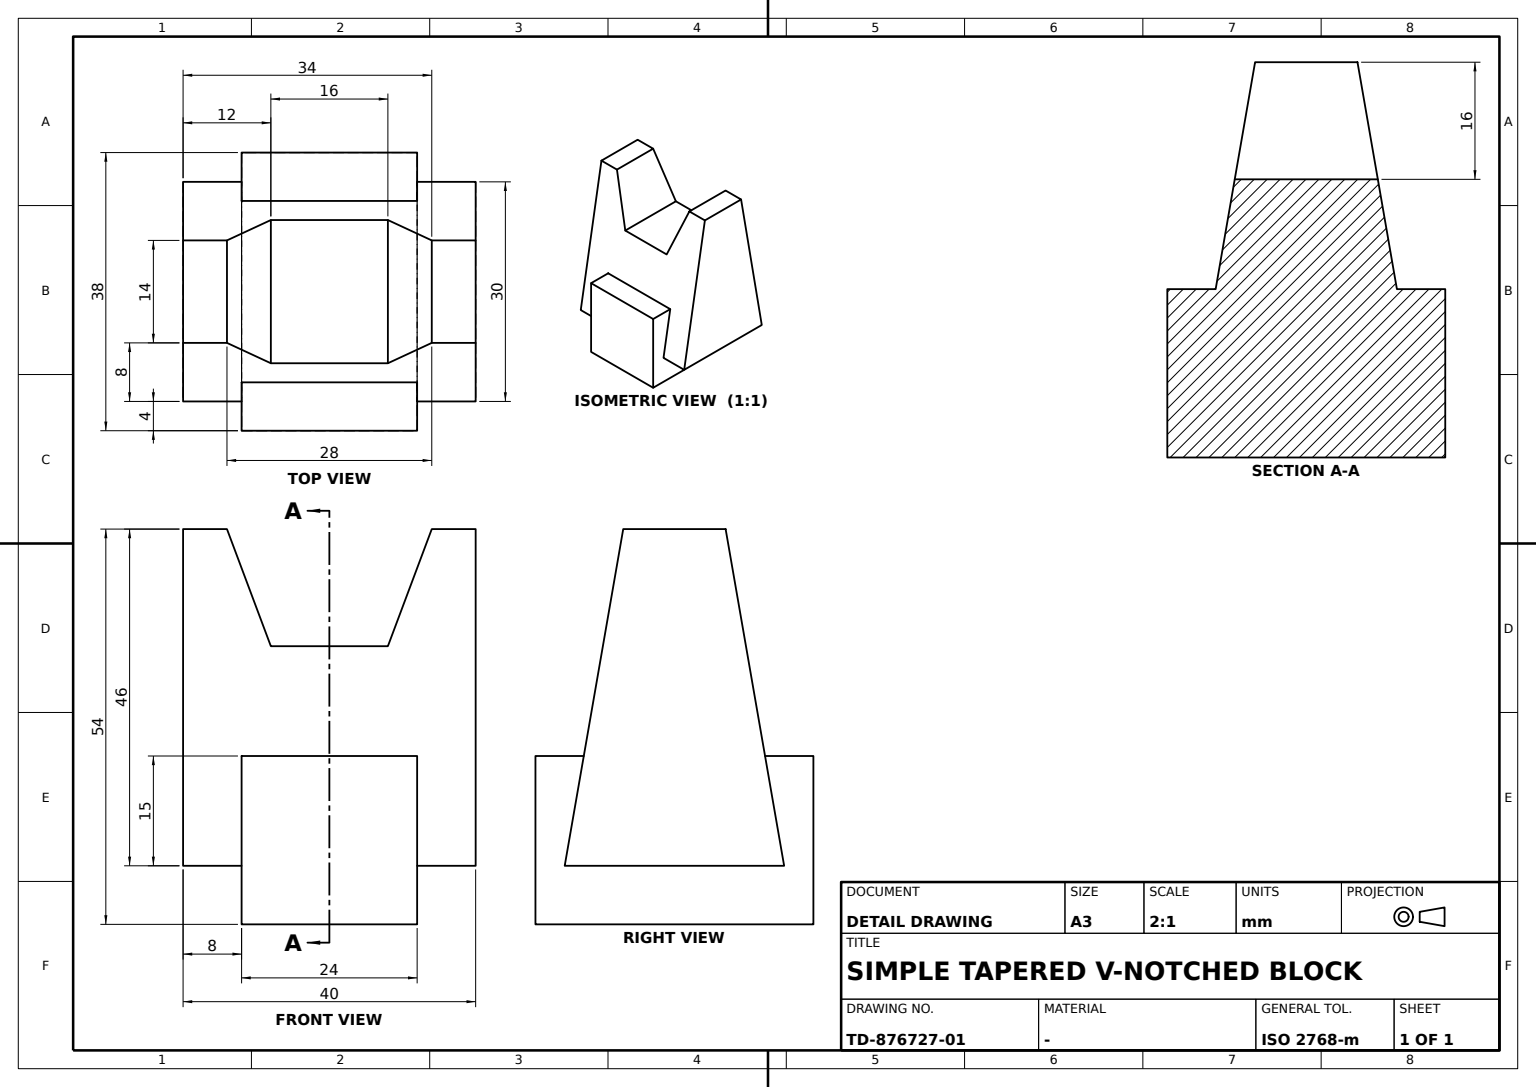
CATIA V5 part; units mm, degrees
sketch "Sketch1" plane through (0, 0, 0) normal (1, 0, 0) x (0, 1, 0)
  point P0 (-12, 0)
  line L0 (-12, 15) -> (12, 15)
  point P1 (14, 0)
  line L1 (14, 0) -> (12, 0)
  point P2 (-12, 0)
  line L2 (-12, 0) -> (-20, 0)
  point P3 (-20, 0)
  line L3 (-20, 0) -> (-20, 46)
  line L4 (-20, 46) -> (-14, 46)
  point P4 (-14, 46)
  line L5 (-14, 46) -> (-8, 30)
  point P5 (-8, 30)
  line L6 (-8, 30) -> (8, 30)
  point P6 (8, 30)
  line L7 (8, 30) -> (14, 46)
  point P7 (14, 46)
  line L8 (14, 46) -> (20, 46)
  line L9 (20, 46) -> (20, 0)
  point P8 (20, 0)
  line L10 (20, 0) -> (14, 0)
  point P9 (14, 0)
  line L11 (-12, 15) -> (-12, 0)
  line L12 (12, 15) -> (12, 0)
  dimension "length L6" = 16
  dimension "distance L4 P5" = 16
  dimension "distance P7 P4" = 28
  dimension "distance L1 L8" = 46
  dimension "distance P3 P8" = 40
  dimension "length L0" = 24
  dimension "distance L0 L2" = 15
  constraint coincidence P0 x-axis
  constraint coincidence P1 x-axis
  constraint coincidence P7 L4
  constraint coincidence P8 L2
  constraint coincidence P1 P9
  constraint coincidence P2 P0
  constraint horizontal L0 x-axis
  constraint horizontal L1 x-axis
  constraint horizontal L2 x-axis
  constraint horizontal L4 x-axis
  constraint horizontal L6 x-axis
  constraint horizontal L8 x-axis
  constraint horizontal L10 x-axis
  constraint vertical L3 y-axis
  constraint vertical L9 y-axis
  constraint vertical L11 y-axis
  constraint vertical L12 y-axis
  constraint symmetry L9 L3 y-axis
  constraint symmetry P5 P6 y-axis
  constraint symmetry L7 L5 y-axis
  constraint symmetry L11 L12 y-axis
extrude "Pad1" add sketch "Sketch1" along normal mid plane 30
sketch "Sketch2" plane through (0, 0, 0) normal (0, 1, 0) x (-1, 0, 0)
  point P0 (-15, 46)
  line L0 (-15, 46) -> (-15, 0)
  point P1 (-15, 0)
  line L1 (-15, 0) -> (-7, 46)
  point P2 (-7, 46)
  line L2 (-7, 46) -> (-15, 46)
  point P3 (7, 46)
  point P4 (15, 0)
  line L3 (15, 0) -> (7, 46)
  point P5 (15, 46)
  line L4 (15, 46) -> (15, 0)
  line L5 (7, 46) -> (15, 46)
  dimension "distance P2 P3" = 14
  dimension "length L2" = 8
  dimension "length L0" = 46
  constraint vertical L0 y-axis
  constraint horizontal L2 x-axis
  constraint coincidence P1 x-axis
  constraint symmetry P2 P3 y-axis
  constraint symmetry P1 P4 y-axis
  constraint symmetry L1 L3 y-axis
  constraint symmetry P0 P5 y-axis
  constraint symmetry L0 L4 y-axis
  constraint symmetry L2 L5 y-axis
extrude "Pocket1" cut sketch "Sketch2" along normal mid plane 66
sketch "Sketch3" plane through (0, 0, 0) normal (1, 0, 0) x (0, 1, 0)
  line L0 (-12, 15) -> (12, 15)
  line L1 (12, 15) -> (12, -8)
  line L2 (12, -8) -> (-12, -8)
  line L3 (-12, -8) -> (-12, 15)
  line L4 (12, 0) -> (12, 15) construction
  line L5 (-12, 0) -> (-12, 15) construction
  line L6 (-12, 15) -> (12, 15) construction
  point P0 (14, 0)
  dimension "distance P0 L2" = 8
  constraint horizontal L0 x-axis
  constraint horizontal L2 x-axis
  constraint vertical L1 y-axis
  constraint vertical L3 y-axis
  constraint coincidence L1 L4
  constraint coincidence L3 L5
  constraint coincidence L0 L6
extrude "Pad2" add sketch "Sketch3" along normal mid plane 38
